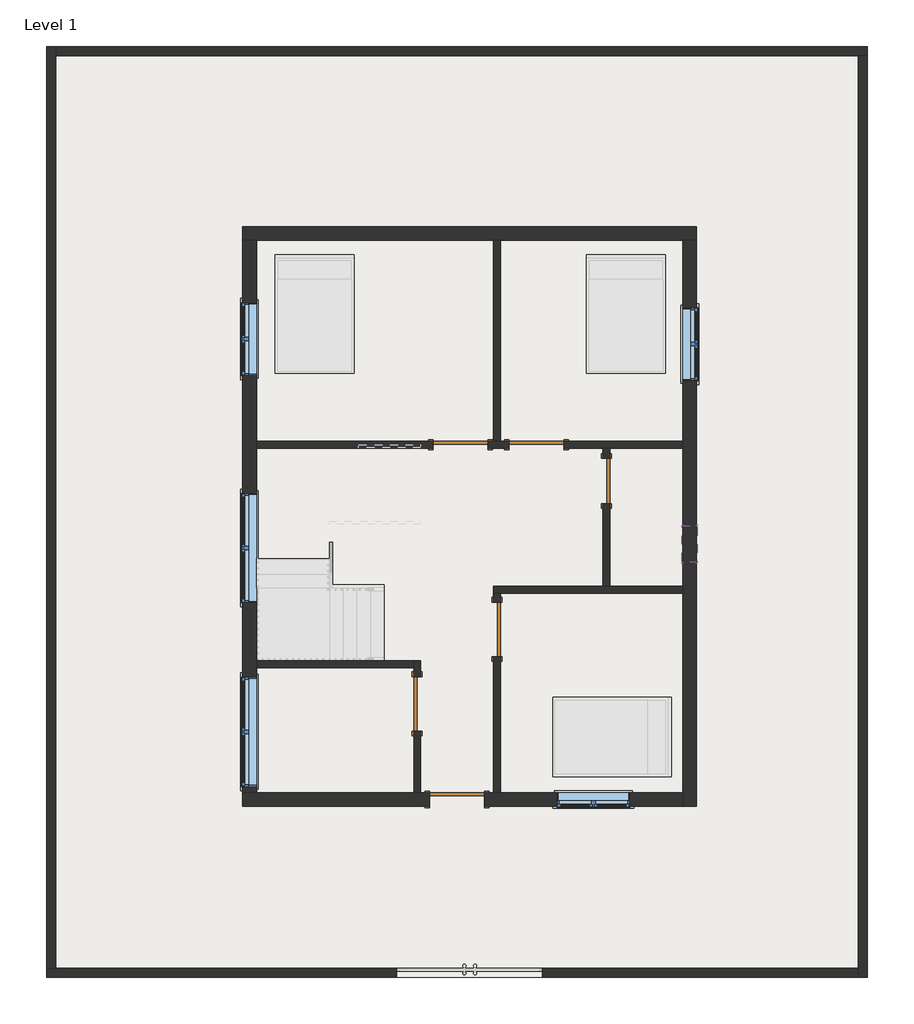
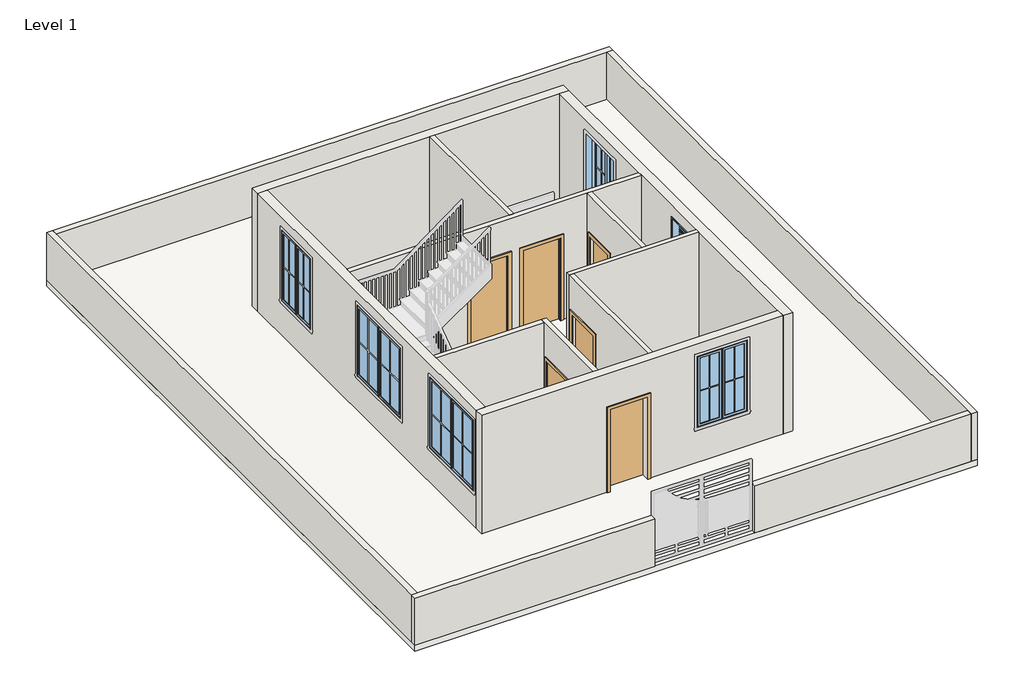
# One storey, part 1 of 3: 16 walls, 6 doors, 6 windows, 1 slab.
"""IFC4 building model written with IfcOpenShell, lengths in millimetres."""

from ifc_helpers import new_model, si_unit, frame, origin, origin_with_axes, place, context, project, spatial, polyline, outline, extrude, faceted_brep, transform, mapped, element, save
from components import door_f2b275c1, single_flush_door_3_e5f9f3c4, single_flush_door_3_305aa2a5, single_flush_door_3_a90ba1ad, window_casement_double_win_4_6ca1769e, window_casement_double_win_6_ce442eab, window_f2d8fef0

model = new_model("IFC4")

# Units and contexts
model_context = context("Model", 3, world=origin())
ifc_project = project(units=[si_unit("LENGTHUNIT", "METRE", prefix="MILLI")], contexts=[model_context])

# Site, building, storey
site = spatial("IfcSite", under=ifc_project)
building = spatial("IfcBuilding", under=site)
storey = spatial("IfcBuildingStorey", under=building, Name="Level 1", Elevation=0.0)

# Doors
placement = place(None, origin())
door_shape = door_f2b275c1(model_context)
element("IfcDoor", 1, ObjectType="Single-Flush : 2'6\"", at=placement, inside=storey, context=model_context, shape_type="MappedRepresentation", body=[
    mapped(door_shape, transform((1031.6394609, 262.5126239, 0.0), x_axis=(0.0, 1.0, 0.0), y_axis=(-1.0, 0.0, 0.0), z_axis=(0.0, 0.0, 1.0))),
])
single_flush_door_3_shape = single_flush_door_3_e5f9f3c4(model_context)
element("IfcDoor", 2, ObjectType="Single-Flush : door 3'", at=placement, inside=storey, context=model_context, shape_type="MappedRepresentation", body=[
    mapped(single_flush_door_3_shape, transform((-1406.7605391, 872.1126239, 0.0), x_axis=(1.0, 0.0, 0.0), y_axis=(0.0, 1.0, 0.0), z_axis=(0.0, 0.0, 1.0))),
])
element("IfcDoor", 3, ObjectType="Single-Flush : door 3'", at=placement, inside=storey, context=model_context, shape_type="MappedRepresentation", body=[
    mapped(single_flush_door_3_shape, transform((-2130.6605391, -3458.5873761, 0.0), x_axis=(0.0, 1.0, 0.0), y_axis=(-1.0, 0.0, 0.0), z_axis=(0.0, 0.0, 1.0))),
])
single_flush_door_3_2_shape = single_flush_door_3_305aa2a5(model_context)
element("IfcDoor", 4, ObjectType="Single-Flush : door 3'", at=placement, inside=storey, context=model_context, shape_type="MappedRepresentation", body=[
    mapped(single_flush_door_3_2_shape, transform((-136.7605391, 872.1126239, 0.0), x_axis=(-1.0, 0.0, 0.0), y_axis=(0.0, -1.0, 0.0), z_axis=(0.0, 0.0, 1.0))),
])
element("IfcDoor", 5, ObjectType="Single-Flush : door 3'", at=placement, inside=storey, context=model_context, shape_type="MappedRepresentation", body=[
    mapped(single_flush_door_3_2_shape, transform((-797.1605391, -2213.9873761, 0.0), x_axis=(0.0, 1.0, 0.0), y_axis=(-1.0, 0.0, 0.0), z_axis=(0.0, 0.0, 1.0))),
])
single_flush_door_3_3_shape = single_flush_door_3_a90ba1ad(model_context)
element("IfcDoor", 6, ObjectType="Single-Flush : door 3'", at=placement, inside=storey, context=model_context, shape_type="MappedRepresentation", body=[
    mapped(single_flush_door_3_3_shape, transform((-1463.9105391, -5052.4373761, 0.0), x_axis=(-1.0, 0.0, 0.0), y_axis=(0.0, -1.0, 0.0), z_axis=(0.0, 0.0, 1.0))),
])

# Slab
element("IfcSlab", 7, ObjectType="floor 6\"", at=placement, inside=storey, context=model_context, shape_type="SweptSolid", body=[
    extrude(outline(polyline([(5391.8596643, 7518.7893563), (5391.8596643, -8026.0106437), (-8324.1403357, -8026.0106437), (-8324.1403357, 7518.7893563), (5391.8596643, 7518.7893563)])), frame((0.0, 0.0, -152.4), z_axis=(0.0, 0.0, 1.0), x_axis=(1.0, 0.0, 0.0)), (0.0, 0.0, 1.0), 152.4),
])

# Walls
element("IfcWall", 8, at=placement, inside=storey, context=model_context, shape_type="Brep", body=[
    faceted_brep([(-8171.7403357, 7366.3893563, 0.0), (5239.4596643, 7366.3893563, 0.0), (5391.8596643, 7366.3893563, 0.0), (5391.8596643, 7366.3893563, 1219.2), (5239.4596643, 7366.3893563, 1219.2), (-8171.7403357, 7366.3893563, 1219.2), (-8171.7403357, 7518.7893563, 0.0), (-8171.7403357, 7518.7893563, 1219.2), (5391.8596643, 7518.7893563, 1219.2), (5391.8596643, 7518.7893563, 0.0)], [[[0, 1, 2, 3, 4, 5]], [[6, 7, 8, 9]], [[2, 1, 0, 6, 9]], [[5, 4, 3, 8, 7]], [[3, 2, 9, 8]], [[0, 5, 7, 6]]]),
])
element("IfcWall", 9, at=placement, inside=storey, context=model_context, shape_type="Brep", body=[
    faceted_brep([(5239.4596643, 7366.3893563, 0.0), (5239.4596643, -7873.6106437, 0.0), (5239.4596643, -8026.0106437, 0.0), (5239.4596643, -8026.0106437, 1219.2), (5239.4596643, -7873.6106437, 1219.2), (5239.4596643, 7366.3893563, 1219.2), (5391.8596643, 7366.3893563, 0.0), (5391.8596643, 7366.3893563, 1219.2), (5391.8596643, -8026.0106437, 1219.2), (5391.8596643, -8026.0106437, 0.0)], [[[0, 1, 2, 3, 4, 5]], [[6, 7, 8, 9]], [[2, 1, 0, 6, 9]], [[5, 4, 3, 8, 7]], [[0, 5, 7, 6]], [[3, 2, 9, 8]]]),
])
element("IfcWall", 10, at=placement, inside=storey, context=model_context, shape_type="SweptSolid", body=[
    extrude(outline(polyline([(-35.1605391, -7873.6106437), (5239.4596643, -7873.6106437), (5239.4596643, -8026.0106437), (-35.1605391, -8026.0106437), (-35.1605391, -7873.6106437)])), origin_with_axes(), (0.0, 0.0, 1.0), 1219.2),
])
element("IfcWall", 11, at=placement, inside=storey, context=model_context, shape_type="Brep", body=[
    faceted_brep([(-8171.7403357, -7873.6106437, 0.0), (-8171.7403357, 7366.3893563, 0.0), (-8171.7403357, 7518.7893563, 0.0), (-8171.7403357, 7518.7893563, 1219.2), (-8171.7403357, 7366.3893563, 1219.2), (-8171.7403357, -7873.6106437, 1219.2), (-8324.1403357, -7873.6106437, 0.0), (-8324.1403357, -7873.6106437, 1219.2), (-8324.1403357, 7518.7893563, 1219.2), (-8324.1403357, 7518.7893563, 0.0)], [[[0, 1, 2, 3, 4, 5]], [[6, 7, 8, 9]], [[2, 1, 0, 6, 9]], [[5, 4, 3, 8, 7]], [[0, 5, 7, 6]], [[3, 2, 9, 8]]]),
])
element("IfcWall", 12, at=placement, inside=storey, context=model_context, shape_type="Brep", body=[
    faceted_brep([(-2473.5605391, -7873.6106437, 0.0), (-8171.7403357, -7873.6106437, 0.0), (-8324.1403357, -7873.6106437, 0.0), (-8324.1403357, -7873.6106437, 1219.2), (-8171.7403357, -7873.6106437, 1219.2), (-2473.5605391, -7873.6106437, 1219.2), (-2473.5605391, -8026.0106437, 0.0), (-2473.5605391, -8026.0106437, 1219.2), (-8324.1403357, -8026.0106437, 1219.2), (-8324.1403357, -8026.0106437, 0.0)], [[[0, 1, 2, 3, 4, 5]], [[6, 7, 8, 9]], [[2, 1, 0, 6, 9]], [[5, 4, 3, 8, 7]], [[0, 5, 7, 6]], [[3, 2, 9, 8]]]),
])
element("IfcWall", 13, ObjectType="WALL 4.5\"", at=placement, inside=storey, context=model_context, shape_type="SweptSolid", body=[
    extrude(outline(polyline([(-854.3105391, 929.2626239), (-854.3105391, 4282.0626239), (-740.0105391, 4282.0626239), (-740.0105391, 929.2626239), (-854.3105391, 929.2626239)])), origin_with_axes(), (0.0, 0.0, 1.0), 3048.0),
])
element("IfcWall", 14, ObjectType="WALL 4.5\"", at=placement, inside=storey, context=model_context, shape_type="Brep", body=[
    faceted_brep([(-949.5605391, 814.9626239, 0.0), (-593.9605391, 814.9626239, 0.0), (-593.9605391, 814.9626239, 2133.6), (320.4394609, 814.9626239, 2133.6), (320.4394609, 814.9626239, 0.0), (974.4894609, 814.9626239, 0.0), (1088.7894609, 814.9626239, 0.0), (2307.9894609, 814.9626239, 0.0), (2307.9894609, 814.9626239, 3048.0), (1088.7894609, 814.9626239, 3048.0), (974.4894609, 814.9626239, 3048.0), (-4816.7105391, 814.9626239, 3048.0), (-4816.7105391, 814.9626239, 0.0), (-1863.9605391, 814.9626239, 0.0), (-1863.9605391, 814.9626239, 2133.6), (-949.5605391, 814.9626239, 2133.6), (-593.9605391, 929.2626239, 2133.6), (-593.9605391, 929.2626239, 0.0), (-740.0105391, 929.2626239, 0.0), (-854.3105391, 929.2626239, 0.0), (-949.5605391, 929.2626239, 0.0), (-949.5605391, 929.2626239, 2133.6), (-1863.9605391, 929.2626239, 2133.6), (-1863.9605391, 929.2626239, 0.0), (-4816.7105391, 929.2626239, 0.0), (-4816.7105391, 929.2626239, 3048.0), (-854.3105391, 929.2626239, 3048.0), (-740.0105391, 929.2626239, 3048.0), (2307.9894609, 929.2626239, 3048.0), (2307.9894609, 929.2626239, 0.0), (320.4394609, 929.2626239, 0.0), (320.4394609, 929.2626239, 2133.6)], [[[0, 1, 2, 3, 4, 5, 6, 7, 8, 9, 10, 11, 12, 13, 14, 15]], [[16, 17, 18, 19, 20, 21, 22, 23, 24, 25, 26, 27, 28, 29, 30, 31]], [[13, 12, 24, 23]], [[30, 29, 7, 6, 5, 4]], [[20, 19, 18, 17, 1, 0]], [[8, 7, 29, 28]], [[12, 11, 25, 24]], [[21, 20, 0, 15]], [[22, 21, 15, 14]], [[23, 22, 14, 13]], [[2, 1, 17, 16]], [[3, 2, 16, 31]], [[4, 3, 31, 30]], [[11, 10, 9, 8, 28, 27, 26, 25]]]),
])
element("IfcWall", 15, ObjectType="WALL 4.5\"", at=placement, inside=storey, context=model_context, shape_type="SweptSolid", body=[
    extrude(outline(polyline([(814.9626239, 0.0), (643.5126239, 0.0), (643.5126239, 2032.0), (-118.4873761, 2032.0), (-118.4873761, 0.0), (-1496.4373761, 0.0), (-1496.4373761, 3048.0), (814.9626239, 3048.0), (814.9626239, 0.0)])), frame((974.4894609, 0.0, 0.0), z_axis=(1.0, 0.0, 0.0), x_axis=(0.0, 1.0, 0.0)), (0.0, 0.0, 1.0), 114.3),
])
element("IfcWall", 16, ObjectType="WALL 4.5\"", at=placement, inside=storey, context=model_context, shape_type="Brep", body=[
    faceted_brep([(2307.9894609, -1496.4373761, 0.0), (1088.7894609, -1496.4373761, 0.0), (974.4894609, -1496.4373761, 0.0), (-854.3105391, -1496.4373761, 0.0), (-854.3105391, -1496.4373761, 3048.0), (974.4894609, -1496.4373761, 3048.0), (1088.7894609, -1496.4373761, 3048.0), (2307.9894609, -1496.4373761, 3048.0), (2307.9894609, -1610.7373761, 0.0), (2307.9894609, -1610.7373761, 3048.0), (-740.0105391, -1610.7373761, 3048.0), (-854.3105391, -1610.7373761, 3048.0), (-854.3105391, -1610.7373761, 0.0), (-740.0105391, -1610.7373761, 0.0)], [[[0, 1, 2, 3, 4, 5, 6, 7]], [[8, 9, 10, 11, 12, 13]], [[3, 2, 1, 0, 8, 13, 12]], [[0, 7, 9, 8]], [[4, 3, 12, 11]], [[7, 6, 5, 4, 11, 10, 9]]]),
])
element("IfcWall", 17, ObjectType="WALL 4.5\"", at=placement, inside=storey, context=model_context, shape_type="SweptSolid", body=[
    extrude(outline(polyline([(-1610.7373761, 0.0), (-1756.7873761, 0.0), (-1756.7873761, 2133.6), (-2671.1873761, 2133.6), (-2671.1873761, 0.0), (-4938.1373761, 0.0), (-4938.1373761, 3048.0), (-1610.7373761, 3048.0), (-1610.7373761, 0.0)])), frame((-854.3105391, 0.0, 0.0), z_axis=(1.0, 0.0, 0.0), x_axis=(0.0, 1.0, 0.0)), (0.0, 0.0, 1.0), 114.3),
])
element("IfcWall", 18, ObjectType="WALL 4.5\"", at=placement, inside=storey, context=model_context, shape_type="Brep", body=[
    faceted_brep([(-2073.5105391, -3001.3873761, 2133.6), (-2073.5105391, -3001.3873761, 0.0), (-2073.5105391, -2741.0373761, 0.0), (-2073.5105391, -2741.0373761, 3048.0), (-2073.5105391, -4938.1373761, 3048.0), (-2073.5105391, -4938.1373761, 0.0), (-2073.5105391, -3915.7873761, 0.0), (-2073.5105391, -3915.7873761, 2133.6), (-2187.8105391, -2741.0373761, 0.0), (-2187.8105391, -2855.3373761, 0.0), (-2187.8105391, -3001.3873761, 0.0), (-2187.8105391, -3001.3873761, 2133.6), (-2187.8105391, -3915.7873761, 2133.6), (-2187.8105391, -3915.7873761, 0.0), (-2187.8105391, -4938.1373761, 0.0), (-2187.8105391, -4938.1373761, 3048.0), (-2187.8105391, -2855.3373761, 3048.0), (-2187.8105391, -2741.0373761, 3048.0)], [[[0, 1, 2, 3, 4, 5, 6, 7]], [[8, 9, 10, 11, 12, 13, 14, 15, 16, 17]], [[6, 5, 14, 13]], [[2, 1, 10, 9, 8]], [[5, 4, 15, 14]], [[3, 2, 8, 17]], [[11, 10, 1, 0]], [[12, 11, 0, 7]], [[13, 12, 7, 6]], [[4, 3, 17, 16, 15]]]),
])
element("IfcWall", 19, ObjectType="WALL 4.5\"", at=placement, inside=storey, context=model_context, shape_type="SweptSolid", body=[
    extrude(outline(polyline([(-4816.7105391, -2741.0373761), (-2187.8105391, -2741.0373761), (-2187.8105391, -2855.3373761), (-4816.7105391, -2855.3373761), (-4816.7105391, -2741.0373761)])), origin_with_axes(), (0.0, 0.0, 1.0), 3048.0),
])
element("IfcWall", 20, ObjectType="WALL 9\"", at=placement, inside=storey, context=model_context, shape_type="Brep", body=[
    faceted_brep([(-5045.3105391, 4282.0626239, 0.0), (-4816.7105391, 4282.0626239, 0.0), (-854.3105391, 4282.0626239, 0.0), (-740.0105391, 4282.0626239, 0.0), (2307.9894609, 4282.0626239, 0.0), (2536.5894609, 4282.0626239, 0.0), (2536.5894609, 4282.0626239, 3048.0), (2307.9894609, 4282.0626239, 3048.0), (-740.0105391, 4282.0626239, 3048.0), (-854.3105391, 4282.0626239, 3048.0), (-4816.7105391, 4282.0626239, 3048.0), (-5045.3105391, 4282.0626239, 3048.0), (-5045.3105391, 4510.6626239, 0.0), (-5045.3105391, 4510.6626239, 3048.0), (2536.5894609, 4510.6626239, 3048.0), (2536.5894609, 4510.6626239, 0.0)], [[[0, 1, 2, 3, 4, 5, 6, 7, 8, 9, 10, 11]], [[12, 13, 14, 15]], [[5, 4, 3, 2, 1, 0, 12, 15]], [[6, 5, 15, 14]], [[0, 11, 13, 12]], [[11, 10, 9, 8, 7, 6, 14, 13]]]),
])
element("IfcWall", 21, ObjectType="WALL 9\"", at=placement, inside=storey, context=model_context, shape_type="Brep", body=[
    faceted_brep([(2307.9894609, 4282.0626239, 0.0), (2307.9894609, 929.2626239, 0.0), (2307.9894609, 814.9626239, 0.0), (2307.9894609, -1496.4373761, 0.0), (2307.9894609, -1610.7373761, 0.0), (2307.9894609, -4938.1373761, 0.0), (2307.9894609, -5166.7373761, 0.0), (2307.9894609, -5166.7373761, 3048.0), (2307.9894609, -4938.1373761, 3048.0), (2307.9894609, -1610.7373761, 3048.0), (2307.9894609, -1496.4373761, 3048.0), (2307.9894609, 814.9626239, 3048.0), (2307.9894609, 929.2626239, 3048.0), (2307.9894609, 4282.0626239, 3048.0), (2307.9894609, 1938.9126239, 2743.2), (2307.9894609, 1938.9126239, 914.4), (2307.9894609, 3158.1126239, 914.4), (2307.9894609, 3158.1126239, 2743.2), (2307.9894609, -486.7873761, 2743.2), (2307.9894609, -1096.3873761, 2743.2), (2307.9894609, -1096.3873761, 2133.6), (2307.9894609, -486.7873761, 2133.6), (2536.5894609, 4282.0626239, 0.0), (2536.5894609, 4282.0626239, 3048.0), (2536.5894609, -5166.7373761, 3048.0), (2536.5894609, -5166.7373761, 0.0), (2536.5894609, 1938.9126239, 2743.2), (2536.5894609, 3158.1126239, 2743.2), (2536.5894609, 3158.1126239, 914.4), (2536.5894609, 1938.9126239, 914.4), (2536.5894609, -486.7873761, 2743.2), (2536.5894609, -486.7873761, 2133.6), (2536.5894609, -1096.3873761, 2133.6), (2536.5894609, -1096.3873761, 2743.2)], [[[0, 1, 2, 3, 4, 5, 6, 7, 8, 9, 10, 11, 12, 13], [14, 15, 16, 17], [18, 19, 20, 21]], [[22, 23, 24, 25], [26, 27, 28, 29], [30, 31, 32, 33]], [[6, 5, 4, 3, 2, 1, 0, 22, 25]], [[0, 13, 23, 22]], [[7, 6, 25, 24]], [[15, 14, 26, 29]], [[16, 15, 29, 28]], [[17, 16, 28, 27]], [[14, 17, 27, 26]], [[31, 30, 18, 21]], [[32, 31, 21, 20]], [[33, 32, 20, 19]], [[30, 33, 19, 18]], [[13, 12, 11, 10, 9, 8, 7, 24, 23]]]),
])
element("IfcWall", 22, ObjectType="WALL 9\"", at=placement, inside=storey, context=model_context, shape_type="Brep", body=[
    faceted_brep([(-1921.1105391, -4938.1373761, 2133.6), (-1921.1105391, -4938.1373761, 0.0), (-2073.5105391, -4938.1373761, 0.0), (-2187.8105391, -4938.1373761, 0.0), (-4816.7105391, -4938.1373761, 0.0), (-5045.3105391, -4938.1373761, 0.0), (-5045.3105391, -4938.1373761, 3048.0), (-4816.7105391, -4938.1373761, 3048.0), (-2187.8105391, -4938.1373761, 3048.0), (-2073.5105391, -4938.1373761, 3048.0), (-854.3105391, -4938.1373761, 3048.0), (-740.0105391, -4938.1373761, 3048.0), (2307.9894609, -4938.1373761, 3048.0), (2307.9894609, -4938.1373761, 0.0), (-740.0105391, -4938.1373761, 0.0), (-854.3105391, -4938.1373761, 0.0), (-1006.7105391, -4938.1373761, 0.0), (-1006.7105391, -4938.1373761, 2133.6), (202.9644609, -4938.1373761, 2743.2), (202.9644609, -4938.1373761, 914.4), (1422.1644609, -4938.1373761, 914.4), (1422.1644609, -4938.1373761, 2743.2), (-5045.3105391, -5166.7373761, 0.0), (-1921.1105391, -5166.7373761, 0.0), (-1921.1105391, -5166.7373761, 2133.6), (-1006.7105391, -5166.7373761, 2133.6), (-1006.7105391, -5166.7373761, 0.0), (2307.9894609, -5166.7373761, 0.0), (2307.9894609, -5166.7373761, 3048.0), (-5045.3105391, -5166.7373761, 3048.0), (202.9644609, -5166.7373761, 2743.2), (1422.1644609, -5166.7373761, 2743.2), (1422.1644609, -5166.7373761, 914.4), (202.9644609, -5166.7373761, 914.4)], [[[0, 1, 2, 3, 4, 5, 6, 7, 8, 9, 10, 11, 12, 13, 14, 15, 16, 17], [18, 19, 20, 21]], [[22, 23, 24, 25, 26, 27, 28, 29], [30, 31, 32, 33]], [[5, 4, 3, 2, 1, 23, 22]], [[16, 15, 14, 13, 27, 26]], [[13, 12, 28, 27]], [[6, 5, 22, 29]], [[19, 18, 30, 33]], [[20, 19, 33, 32]], [[21, 20, 32, 31]], [[18, 21, 31, 30]], [[24, 23, 1, 0]], [[25, 24, 0, 17]], [[26, 25, 17, 16]], [[12, 11, 10, 9, 8, 7, 6, 29, 28]]]),
])
element("IfcWall", 23, ObjectType="WALL 9\"", at=placement, inside=storey, context=model_context, shape_type="Brep", body=[
    faceted_brep([(-4816.7105391, -4938.1373761, 0.0), (-4816.7105391, -2855.3373761, 0.0), (-4816.7105391, -2741.0373761, 0.0), (-4816.7105391, 814.9626239, 0.0), (-4816.7105391, 929.2626239, 0.0), (-4816.7105391, 4282.0626239, 0.0), (-4816.7105391, 4282.0626239, 3048.0), (-4816.7105391, 929.2626239, 3048.0), (-4816.7105391, 814.9626239, 3048.0), (-4816.7105391, -2741.0373761, 3048.0), (-4816.7105391, -2855.3373761, 3048.0), (-4816.7105391, -4938.1373761, 3048.0), (-4816.7105391, -3010.9123761, 2743.2), (-4816.7105391, -3010.9123761, 914.4), (-4816.7105391, -4839.7123761, 914.4), (-4816.7105391, -4839.7123761, 2743.2), (-4816.7105391, 59.3126239, 2743.2), (-4816.7105391, 59.3126239, 914.4), (-4816.7105391, -1769.4873761, 914.4), (-4816.7105391, -1769.4873761, 2743.2), (-4816.7105391, 3243.8376239, 2743.2), (-4816.7105391, 3243.8376239, 914.4), (-4816.7105391, 2024.6376239, 914.4), (-4816.7105391, 2024.6376239, 2743.2), (-5045.3105391, -4938.1373761, 0.0), (-5045.3105391, -4938.1373761, 3048.0), (-5045.3105391, 4282.0626239, 3048.0), (-5045.3105391, 4282.0626239, 0.0), (-5045.3105391, -3010.9123761, 2743.2), (-5045.3105391, -4839.7123761, 2743.2), (-5045.3105391, -4839.7123761, 914.4), (-5045.3105391, -3010.9123761, 914.4), (-5045.3105391, 59.3126239, 2743.2), (-5045.3105391, -1769.4873761, 2743.2), (-5045.3105391, -1769.4873761, 914.4), (-5045.3105391, 59.3126239, 914.4), (-5045.3105391, 3243.8376239, 2743.2), (-5045.3105391, 2024.6376239, 2743.2), (-5045.3105391, 2024.6376239, 914.4), (-5045.3105391, 3243.8376239, 914.4)], [[[0, 1, 2, 3, 4, 5, 6, 7, 8, 9, 10, 11], [12, 13, 14, 15], [16, 17, 18, 19], [20, 21, 22, 23]], [[24, 25, 26, 27], [28, 29, 30, 31], [32, 33, 34, 35], [36, 37, 38, 39]], [[5, 4, 3, 2, 1, 0, 24, 27]], [[6, 5, 27, 26]], [[0, 11, 25, 24]], [[13, 12, 28, 31]], [[14, 13, 31, 30]], [[15, 14, 30, 29]], [[12, 15, 29, 28]], [[17, 16, 32, 35]], [[18, 17, 35, 34]], [[19, 18, 34, 33]], [[16, 19, 33, 32]], [[21, 20, 36, 39]], [[22, 21, 39, 38]], [[23, 22, 38, 37]], [[20, 23, 37, 36]], [[11, 10, 9, 8, 7, 6, 26, 25]]]),
])

# Windows
window_casement_double_win_4_shape = window_casement_double_win_4_6ca1769e(model_context)
element("IfcWindow", 24, ObjectType="Window-Casement-Double : win 4'", at=placement, inside=storey, context=model_context, shape_type="MappedRepresentation", body=[
    mapped(window_casement_double_win_4_shape, transform((812.5644609, -5052.4373761, 0.0), x_axis=(-1.0, 0.0, 0.0), y_axis=(0.0, -1.0, 0.0), z_axis=(0.0, 0.0, 1.0))),
])
element("IfcWindow", 25, ObjectType="Window-Casement-Double : win 4'", at=placement, inside=storey, context=model_context, shape_type="MappedRepresentation", body=[
    mapped(window_casement_double_win_4_shape, transform((2422.2894609, 2548.5126239, 0.0), x_axis=(0.0, -1.0, 0.0), y_axis=(1.0, 0.0, 0.0), z_axis=(0.0, 0.0, 1.0))),
])
element("IfcWindow", 26, ObjectType="Window-Casement-Double : win 4'", at=placement, inside=storey, context=model_context, shape_type="MappedRepresentation", body=[
    mapped(window_casement_double_win_4_shape, transform((-4931.0105391, 2634.2376239, 0.0), x_axis=(0.0, 1.0, 0.0), y_axis=(-1.0, 0.0, 0.0), z_axis=(0.0, 0.0, 1.0))),
])
window_casement_double_win_6_shape = window_casement_double_win_6_ce442eab(model_context)
element("IfcWindow", 27, ObjectType="Window-Casement-Double : win 6'", at=placement, inside=storey, context=model_context, shape_type="MappedRepresentation", body=[
    mapped(window_casement_double_win_6_shape, transform((-4931.0105391, -3925.3123761, 0.0), x_axis=(0.0, 1.0, 0.0), y_axis=(-1.0, 0.0, 0.0), z_axis=(0.0, 0.0, 1.0))),
])
element("IfcWindow", 28, ObjectType="Window-Casement-Double : win 6'", at=placement, inside=storey, context=model_context, shape_type="MappedRepresentation", body=[
    mapped(window_casement_double_win_6_shape, transform((-4931.0105391, -855.0873761, 0.0), x_axis=(0.0, 1.0, 0.0), y_axis=(-1.0, 0.0, 0.0), z_axis=(0.0, 0.0, 1.0))),
])
window_shape = window_f2d8fef0(model_context)
element("IfcWindow", 29, ObjectType="Window-Louvers : 24\" x 24\"", at=placement, inside=storey, context=model_context, shape_type="MappedRepresentation", body=[
    mapped(window_shape, transform((2428.6394609, -791.5873761, 1219.2), x_axis=(0.0, -1.0, 0.0), y_axis=(1.0, 0.0, 0.0), z_axis=(0.0, 0.0, 1.0))),
])

save(model, "model.ifc")

# Revit data of these elements
# Type "Single-Flush : 2'6\""
#   Type Mark = "9"
#   Construction Type Id = "MDOOR"
#   Assembly Code = "C1020"
#   Analytic Construction = "Metal"
#   Thickness = 0' - 2"
#   Heat Transfer Coefficient (U) = 0.651978 BTU/(h·ft²·°F)
#   Height = 6' - 8"
#   Trim Projection Ext = 0' - 1"
#   Trim Projection Int = 0' - 1"
#   Trim Width = 0' - 3"
#   Width = 2' - 6"
#   Define Thermal Properties by = 1
#   Door Material = Door - Panel
#   Frame Material = Door - Frame
#   Visual Light Transmittance = 0
#   Solar Heat Gain Coefficient = 0
#   Function = (empty or 0)
#   Wall Closure = (empty or 0)
# Type "Single-Flush : door 3'"
#   Type Mark = "8"
#   Construction Type Id = "MDOOR"
#   Assembly Code = "C1020"
#   Analytic Construction = "Metal"
#   Thickness = 0' - 2"
#   Heat Transfer Coefficient (U) = 0.651978 BTU/(h·ft²·°F)
#   Height = 7' - 0"
#   Trim Projection Ext = 0' - 1"
#   Trim Projection Int = 0' - 1"
#   Trim Width = 0' - 3"
#   Width = 3' - 0"
#   Define Thermal Properties by = 1
#   Door Material = Door - Panel
#   Frame Material = Door - Frame
#   Visual Light Transmittance = 0
#   Solar Heat Gain Coefficient = 0
#   Function = (empty or 0)
#   Wall Closure = (empty or 0)
# Type "floor 6\""
#   Assembly Code = "B1010"
#   Function = 0
#   Layers, outside or top first: 0' - 6" no material (function 1)
# Type
#   Assembly Code = "B2010"
#   Layers, outside or top first: 0' - 6" no material (function 1)
# Type "WALL 4.5\""
#   Assembly Code = "B2010"
#   Layers, outside or top first: 0' - 4 1/2" no material (function 1)
# Type "WALL 9\""
#   Assembly Code = "B2010"
#   Layers, outside or top first: 0' - 9" no material (function 1)
# Type "Window-Casement-Double : win 4'"
#   Type Mark = "19"
#   Fire Rating = "0.5h"
#   Assembly Code = "B2020100"
#   Analytic Construction = "Double glazing - domestic"
#   Frame Extension [instance default] = 0' - 0 1/4"
#   Window Inset [instance default] = 0' - 0"
#   Wall Thickness [instance default] = 0' - 6"
#   Interior Wall Closure [instance default] = 0' - 2 1/4"
#   Half Width = 2' - 0"
#   Visual Light Transmittance = 0.81
#   Thermal Resistance (R) = 1.8146 (h·ft²·°F)/BTU
#   Solar Heat Gain Coefficient = 0.76
#   Rough Width = 4' - 0 1/2"
#   Rough Height = 6' - 0 1/2"
#   Height = 6' - 0"
#   Heat Transfer Coefficient (U) = 0.5511 BTU/(h·ft²·°F)
#   Exterior Wall Closure [instance default] = 0' - 1 1/4"
#   Extension Jamb [instance default] = 0' - 2 1/4"
#   Default Sill Height = 3' - 0"
#   Width = 4' - 0"
#   Muntin Visibility = yes
#   Interior Trim Visibility [instance default] = yes
#   Exterior Trim Visibility [instance default] = yes
#   Extension Jamb Visibility [instance default] = yes
#   Interior Trim Material = Wood - Stained
#   Muntin Pattern = Muntin Pattern_2x2 : Muntin Pattern_2x2
#   Interior Trim = Trim-Window-Interior-Flat : Picture Frame
#   Interior Frame Material = Wood - Stained
#   Glass Panel Material = Glass
#   Exterior Trim Material = Clad - White
#   Exterior Trim = Trim-Window-Exterior-Flat : with Sill
#   Exterior Frame Material = Clad - White
#   Wall Closure = (empty or 0)
# Type "Window-Casement-Double : win 6'"
#   Type Mark = "18"
#   Fire Rating = "0.5h"
#   Assembly Code = "B2020100"
#   Analytic Construction = "Double glazing - domestic"
#   Frame Extension [instance default] = 0' - 0 1/4"
#   Window Inset [instance default] = 0' - 0"
#   Wall Thickness [instance default] = 0' - 6"
#   Interior Wall Closure [instance default] = 0' - 2 1/4"
#   Half Width = 3' - 0"
#   Visual Light Transmittance = 0.81
#   Thermal Resistance (R) = 1.8146 (h·ft²·°F)/BTU
#   Solar Heat Gain Coefficient = 0.76
#   Rough Width = 6' - 0 1/2"
#   Rough Height = 6' - 0 1/2"
#   Height = 6' - 0"
#   Heat Transfer Coefficient (U) = 0.5511 BTU/(h·ft²·°F)
#   Exterior Wall Closure [instance default] = 0' - 1 1/4"
#   Extension Jamb [instance default] = 0' - 2 1/4"
#   Default Sill Height = 3' - 0"
#   Width = 6' - 0"
#   Muntin Visibility = yes
#   Interior Trim Visibility [instance default] = yes
#   Exterior Trim Visibility [instance default] = yes
#   Extension Jamb Visibility [instance default] = yes
#   Interior Trim Material = Wood - Stained
#   Muntin Pattern = Muntin Pattern_2x2 : Muntin Pattern_2x2
#   Interior Trim = Trim-Window-Interior-Flat : Picture Frame
#   Interior Frame Material = Wood - Stained
#   Glass Panel Material = Glass
#   Exterior Trim Material = Clad - White
#   Exterior Trim = Trim-Window-Exterior-Flat : with Sill
#   Exterior Frame Material = Clad - White
#   Wall Closure = (empty or 0)
# Type "Window-Louvers : 24\" x 24\""
#   Type Mark = "20"
#   Construction Type Id = "GSP4R"
#   Assembly Code = "B20"
#   Analytic Construction = "1/8 in Pilkington single glazing"
#   Visual Light Transmittance = 0.9
#   Thermal Resistance (R) = 1.53941 (h·ft²·°F)/BTU
#   Solar Heat Gain Coefficient = 0.78
#   Max Height = 1' - 11.74264"
#   Height = 2' - 0"
#   Heat Transfer Coefficient (U) = 0.6496 BTU/(h·ft²·°F)
#   Blade Width [instance default] = 1' - 10 1/2"
#   Blade Vertical Thickness = 0' - 0.35355"
#   Blade Thickness = 0' - 0 1/4"
#   Blade Spacing = 0' - 1 1/2"
#   Blade Height = 0' - 1.85355"
#   Blade Depth = 0' - 3"
#   Blade Angle = 45.00°
#   Default Sill Height = 3' - 0"
#   Trim Projection_Exterior = 0' - 0 1/2"
#   Trim Projection_Interior = 0' - 0 1/2"
#   Trim Width_Exterior = 0' - 1 1/2"
#   Trim Width_Interior = 0' - 1 1/2"
#   Width = 2' - 0"
#   Max Blade Count = 12
#   Define Thermal Properties by = 1
#   Blade Count = 12
#   Frame Material = Birch
#   Louver Material = Birch
#   Trim Exterior Material = Birch
#   Trim Interior Material = Birch
#   Wall Closure = (empty or 0)
# Element 1 (IfcDoor, "Single-Flush : 2'6\"")
#   Phase Created = New Construction
#   Materials on its faces: "Door - Frame", "Door - Panel"
# Elements 2, 3, 4, 5, 6 (IfcDoor, "Single-Flush : door 3'")
#   Phase Created = New Construction
#   Materials on its faces: "Door - Frame", "Door - Panel"
# Element 7 (IfcSlab, "floor 6\"")
#   Height Offset From Level = 0' - 0"
#   Phase Created = New Construction
#   Materials on its faces: "Wood Planks", "Default Floor", "Wood - Stained"
# Elements 8, 9, 11 (IfcWall)
#   Top Offset = 0' - 0"
#   Base Offset = 0' - 0"
#   Unconnected Height = 4' - 0"
#   wall height = 4' - 0"
#   Phase Created = New Construction
#   Base Constraint = Level 1
#   Materials on its faces: "Clad - White", "Default Wall", "Wood Planks"
# Element 10 (IfcWall)
#   Top Offset = 0' - 0"
#   Base Offset = 0' - 0"
#   Unconnected Height = 4' - 0"
#   wall height = 4' - 0"
#   Phase Created = New Construction
#   Base Constraint = Level 1
#   Materials on its faces: "Default Wall", "Clad - White", "Wood Planks"
# Element 12 (IfcWall)
#   Top Offset = 0' - 0"
#   Base Offset = 0' - 0"
#   Unconnected Height = 4' - 0"
#   wall height = 4' - 0"
#   Phase Created = New Construction
#   Base Constraint = Level 1
#   Materials on its faces: "Clad - White", "Wood Planks", "Default Wall"
# Elements 13, 14, 15, 16, 17, 18, 19 (IfcWall, "WALL 4.5\"")
#   Top Offset = 0' - 0"
#   Base Offset = 0' - 0"
#   Unconnected Height = 10' - 0"
#   wall height = 10' - 0"
#   Phase Created = New Construction
#   Base Constraint = Level 1
#   Materials on its faces: "Default Wall"
# Elements 20, 21, 22, 23 (IfcWall, "WALL 9\"")
#   Top Offset = 0' - 0"
#   Base Offset = 0' - 0"
#   Unconnected Height = 10' - 0"
#   wall height = 10' - 0"
#   Phase Created = New Construction
#   Base Constraint = Level 1
#   Materials on its faces: "Default Wall", "Door - Frame"
# Element 24 (IfcWindow, "Window-Casement-Double : win 4'")
#   Mark = "3"
#   Window Inset = 0' - 0"
#   Interior Wall Closure = 0' - 2 1/4"
#   Frame Extension = 0' - 0 1/4"
#   Exterior Wall Closure = 0' - 1 1/4"
#   Interior Trim Visibility = yes
#   Exterior Trim Visibility = yes
#   Phase Created = New Construction
#   Materials on its faces: "Wood - Stained", "Glass", "Clad - White"
# Element 25 (IfcWindow, "Window-Casement-Double : win 4'")
#   Mark = "4"
#   Window Inset = 0' - 0"
#   Interior Wall Closure = 0' - 2 1/4"
#   Frame Extension = 0' - 0 1/4"
#   Exterior Wall Closure = 0' - 1 1/4"
#   Interior Trim Visibility = yes
#   Exterior Trim Visibility = yes
#   Phase Created = New Construction
#   Materials on its faces: "Wood - Stained", "Glass", "Clad - White"
# Element 26 (IfcWindow, "Window-Casement-Double : win 4'")
#   Mark = "5"
#   Window Inset = 0' - 0"
#   Interior Wall Closure = 0' - 2 1/4"
#   Frame Extension = 0' - 0 1/4"
#   Exterior Wall Closure = 0' - 1 1/4"
#   Interior Trim Visibility = yes
#   Exterior Trim Visibility = yes
#   Phase Created = New Construction
#   Materials on its faces: "Wood - Stained", "Glass", "Clad - White"
# Element 27 (IfcWindow, "Window-Casement-Double : win 6'")
#   Mark = "1"
#   Window Inset = 0' - 0"
#   Interior Wall Closure = 0' - 2 1/4"
#   Frame Extension = 0' - 0 1/4"
#   Exterior Wall Closure = 0' - 1 1/4"
#   Interior Trim Visibility = yes
#   Exterior Trim Visibility = yes
#   Phase Created = New Construction
#   Materials on its faces: "Wood - Stained", "Glass", "Clad - White"
# Element 28 (IfcWindow, "Window-Casement-Double : win 6'")
#   Mark = "2"
#   Window Inset = 0' - 0"
#   Interior Wall Closure = 0' - 2 1/4"
#   Frame Extension = 0' - 0 1/4"
#   Exterior Wall Closure = 0' - 1 1/4"
#   Interior Trim Visibility = yes
#   Exterior Trim Visibility = yes
#   Phase Created = New Construction
#   Materials on its faces: "Wood - Stained", "Glass", "Clad - White"
# Element 29 (IfcWindow, "Window-Louvers : 24\" x 24\"")
#   Mark = "6"
#   Blade Width = 1' - 10 1/2"
#   Phase Created = New Construction
#   Materials on its faces: "Birch"
# Materials
#   "Door - Panel": class "Wood", colour RGB 210 159 95, transparency 0, Cost = 0
#   "Door - Frame": colour RGB 118 70 51, transparency 0, Cost = 0
#   "Wood - Stained": class "Wood", colour RGB 224 178 126, transparency 0, Cost = 0
#   "Glass": class "Glass", colour RGB 0 128 192, transparency 0.75, Description = "Soda Lime Glass", Cost = 0
#   "Clad - White": class "Wood", colour RGB 242 242 238, transparency 0, Cost = 0
#   "Birch": class "Wood", colour RGB 224 178 126, transparency 0, Description = "Betula Alleghaniensis", Cost = 0
#   "Wood Planks": class "Wood", colour RGB 193 160 115, transparency 0, Description = "Physical material.", Cost = 0
#   "Default Floor": colour RGB 128 128 128, transparency 0, Cost = 0
#   "Default Wall": colour RGB 128 128 128, transparency 0, Cost = 0
